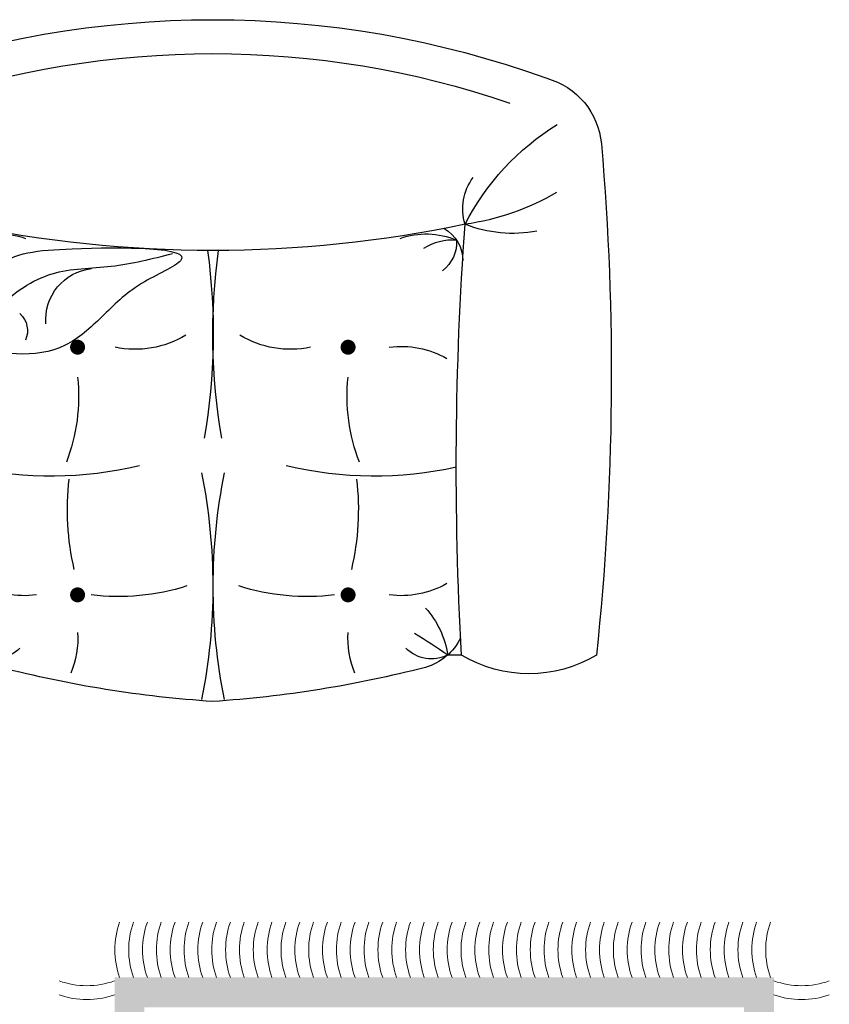
# Model space of a CAD drawing. Units: inches. Extents: x 844 to 2234, y 346 to 1084.
# Tile 63 of 93: x 1860.31 to 1877.53, y 712.91 to 733.85. Entities that reach past the tile are written whole.
import ezdxf

# ---------------------------------------------------------------- set-up
doc = ezdxf.new("R2010")
doc.units = ezdxf.units.IN
doc.header["$MEASUREMENT"] = 0
doc.layers.add('furniture', color=8, linetype='Continuous', lineweight=18)
doc.layers.add('RA-AP-01$0$INT', color=35, linetype='Continuous', lineweight=5)
doc.layers.add('RA-AP-01$0$FURN', color=3, linetype='Continuous')
doc.layers.add('RA-AP-01$0$WOOD', color=64, linetype='Continuous')

# ---------------------------------------------------------------- blocks, each defined once
blk = doc.blocks.new('A$C18D01794')
at = {"layer": 'RA-AP-01$0$INT'}
h = blk.add_hatch(color=256, dxfattribs=at)
h.paths.add_polyline_path([(4.355206456958071, -6.156712009588037), (4.355206456958071, -8.056712009588038), (5.455206456958072, -8.056712009588038), (5.455206456958072, -6.156712009588037)])
h.paths.add_polyline_path([(4.405206456958072, -8.006712009588039), (4.405206456958072, -6.206712009588038), (5.405206456958072, -6.206712009588038), (5.405206456958072, -8.006712009588039)], flags=16)
for centre, start, end in [((4.309006456945037, -8.156264458284674), 70.20384312815696, 109.7961568705686), ((5.501406456971106, -8.156264458284674), 70.20384312943132, 109.796156871843), ((4.309006456945037, -8.179364458283423), 70.20384312815696, 109.7961568705686), ((5.501406456971106, -8.179364458283423), 70.20384312943132, 109.796156871843), ((4.492158905671144, -8.102912009578965), 160.2038431286875, 199.7961568711004), ((4.515258905666937, -8.102912009582035), 160.2038431286875, 199.7961568711004), ((4.53835890566273, -8.102912009585104), 160.2038431286875, 199.7961568711004), ((4.561458905665799, -8.102912009585218), 160.2038431286875, 199.7961568711004), ((4.584558905661592, -8.102912009588287), 160.2038431286875, 199.7961568711004), ((4.607658905664661, -8.102912009588401), 160.2038431286875, 199.7961568711004), ((4.630758905664774, -8.102912009585673), 160.2038431286875, 199.7961568711004), ((4.653858905660567, -8.102912009588742), 160.2038431286875, 199.7961568711004), ((4.676958905663636, -8.102912009588856), 160.2038431286875, 199.7961568711004), ((4.700058905663976, -8.102912009589083), 160.2038431286875, 199.7961568711004), ((4.723158905662498, -8.102912009586241), 160.2038431286875, 199.7961568711004), ((4.746258905662839, -8.102912009586355), 160.2038431286875, 199.7961568711004), ((4.769358905662952, -8.102912009589536), 160.2038431286875, 199.7961568711004), ((4.792458905660109, -8.102912009586696), 160.2038431286875, 199.7961568711004), ((4.815558905661814, -8.10291200958681), 160.2038431286875, 199.7961568711004), ((4.838658905662154, -8.102912009587037), 160.2038431286875, 199.7961568711004), ((4.861758905665223, -8.102912009590106), 160.2038431286875, 199.7961568711004), ((4.884858905661016, -8.102912009587264), 160.2038431286875, 199.7961568711004), ((4.907958905662721, -8.102912009587492), 160.2038431286875, 199.7961568711004), ((4.931058905658514, -8.102912009590447), 160.2038431286875, 199.7961568711004), ((4.954158905661583, -8.102912009587717), 160.2038431286875, 199.7961568711004), ((4.977258905663288, -8.102912009587946), 160.2038431286875, 199.7961568711004), ((5.000358905663628, -8.102912009587946), 160.2038431286875, 199.7961568711004), ((5.023458905665333, -8.10291200959113), 160.2038431286875, 199.7961568711004), ((5.046558905660899, -8.102912009588287), 160.2038431286875, 199.7961568711004), ((5.069658905661239, -8.102912009588401), 160.2038431286875, 199.7961568711004), ((5.092758905664308, -8.102912009588628), 160.2038431286875, 199.7961568711004), ((5.115858905663057, -8.102912009585786), 160.2038431286875, 199.7961568711004), ((5.13895890566317, -8.102912009588856), 160.2038431286875, 199.7961568711004), ((5.162058905663511, -8.102912009589083), 160.2038431286875, 199.7961568711004), ((5.185158905659076, -8.102912009589197), 160.2038431286875, 199.7961568711004), ((5.208258905660781, -8.102912009586355), 160.2038431286875, 199.7961568711004), ((5.231358905662486, -8.102912009589536), 160.2038431286875, 199.7961568711004), ((5.254458905661235, -8.102912009589652), 160.2038431286875, 199.7961568711004), ((5.277558905661575, -8.102912009589765), 160.2038431286875, 199.7961568711004), ((5.300658905661689, -8.102912009587037), 160.2038431286875, 199.7961568711004), ((5.323758905658846, -8.10291200958715), 160.2038431286875, 199.7961568711004), ((5.346858905659186, -8.10291200959022), 160.2038431286875, 199.7961568711004), ((5.369958905662255, -8.102912009587492), 160.2038431286875, 199.7961568711004), ((5.39305890566396, -8.102912009587492), 160.2038431286875, 199.7961568711004), ((5.416158905664301, -8.102912009587717), 160.2038431286875, 199.7961568711004), ((5.439258905666005, -8.102912009590902), 160.2038431286875, 199.7961568711004), ((5.462358905661571, -8.102912009587946), 160.2038431286875, 199.7961568711004), ((5.485458905657364, -8.10291200958499), 160.2038431286875, 199.7961568711004), ((5.508558905660433, -8.102912009588287), 160.2038431286875, 199.7961568711004), ((5.531658905655999, -8.102912009585332), 160.2038431286875, 199.7961568711004), ((5.554758905651792, -8.102912009582376), 160.2038431286875, 199.7961568711004), ((5.577858905654861, -8.102912009585673), 160.2038431286875, 199.7961568711004)]:
    blk.add_arc(centre, 0.136414042854523, start, end, dxfattribs=at)
blk = doc.blocks.new('A$C7F4351E2')
at = {"layer": 'RA-AP-01$0$FURN'}
for p, q in [((8.352559572600457, -8.263941955512525), (8.35255957259913, -8.282283310927069)), ((8.352559572600457, -8.927748273106442), (8.35255957259913, -8.909406917691898))]:
    blk.add_line(p, q, dxfattribs=at)
at = {"layer": 'RA-AP-01$0$FURN', "const_width": 0.01}
for points in [[(8.437812509519787, -8.415359762755768, 1), (8.427812509519786, -8.415359762755742, 1)], [(8.758197489244363, -8.415359762756214, -1), (8.768197489244365, -8.415359762756214, -1)], [(8.437812509519787, -8.776330465863198, -1), (8.427812509519786, -8.776330465863225, -1)], [(8.758197489244363, -8.776330465862753, 1), (8.768197489244365, -8.776330465862753, 1)]]:
    blk.add_lwpolyline(points, format="xyb", close=True, dxfattribs=at)
at = {"layer": 'RA-AP-01$0$FURN'}
for centre, radius, start, end in [((8.727559572604601, -11.61690445537682), 3.552808610866049, 85.0473312316413, 96.05887237565803), ((9.025650106946005, -8.176987401637472), 0.1, 15.499494600857, 85.04733123164159), ((8.50205957259015, -8.17394195551301), 0.1744999999876311, 148.9517780040467, 211.048221995953), ((8.77247054904813, -7.958543863781743), 0.3382138395168437, 297.2303327094027, 328.2563708342649), ((9.2484631175852, -8.302692737637487), 0.3241573581843151, 149.2985674842688, 172.3026350986055), ((7.88981694267423, -8.595845114309485), 1.310286319972027, 340.1192502251003, 19.8807497748998), ((9.084915705374858, -8.196040134964925), 0.1698955038956699, 168.877843135945, 201.8512383801196), ((7.929864357850293, -8.595845114309483), 1.224941341589781, 341.1257460634955, 18.87425393650447), ((8.947672844970796, -8.191835192646359), 0.0704710051510922, 253.1338634205325, 306.4126496157095), ((8.603635103111959, -3.79706073025477), 4.473931917517753, 266.7828902523826, 274.1477233631118), ((10.52713941284929, -8.595845114309466), 1.634931324962266, 168.1200364254424, 191.8799635745573), ((8.408522229993444, -8.33300072568355), 0.0753785023123622, 115.8745619060558, 163.9833547230034), ((9.101231010340802, -8.38034106221356), 0.5100538472773755, 167.6182489359307, 193.3122231353938), ((8.903279781571525, -8.31837865610295), 0.0478550828899777, 86.575295631534, 142.6833829238214), ((8.878389979098333, -8.312202545234353), 0.05, 30.14777190425723, 89.99999999905349), ((8.838100984994732, -8.276822957859652), 0.0683206773889159, 326.6729861493449, 5.218395042636973), ((8.810121490949696, -8.31110757721543), 0.1042084262671507, 340.4828318717155, 22.86929393278168), ((8.395364730619693, -8.304213854581548), 0.0479292786975047, 152.8070868543555, 225.4025460716553), ((8.333592787569726, -8.402663469525104), 0.1218651776285568, 48.0375529564433, 81.04623209541253), ((7.439612310514541, -8.913795367824825), 1.11020813118073, 31.93286085977143, 34.66647731879807), ((8.553131949433, -8.344109762755968), 0.1214118203512435, 150.1419074485596, 187.691663289156), ((8.642878049331348, -8.344109762756093), 0.1214118203512435, 352.3083367106845, 29.85809255128089), ((9.82633505008426, -8.696671375220811), 1.539060359583382, 165.5338783218257, 176.2437734318419), ((8.374918524725835, -8.294321202996931), 0.1212957045587361, 247.3375839744822, 273.7314750942433), ((8.546954810732721, -8.753394424755975), 0.3517162425384579, 83.41248966761125, 103.1674570565571), ((8.697701155637269, -8.172468128267624), 0.2442261434243043, 248.9017070735605, 275.9923925191661), ((8.73287643248165, -8.469775898206471), 0.3023568492824586, 173.0944825511667, 197.588060785551), ((8.889871101981017, -8.492307869305423), 0.1295083186917369, 167.9901339202812, 211.3796151021958), ((8.444145567704187, -7.829943385268752), 0.765467899454341, 258.6273206109321, 281.4174148186357), ((8.781211457338294, -7.772561243483908), 0.8232838708255751, 260.2449188973366, 277.7495311655964), ((9.82633505008426, -8.495018853398156), 1.539060359583382, 183.7562265681581, 194.4661216781742), ((8.444145567704187, -9.361312955433425), 0.765467899454341, 78.58258518136427, 101.3726793890678), ((8.781211457338294, -9.418695097218269), 0.8232838708255751, 82.25060502413102, 99.75508110266344), ((8.73287643248165, -8.721914330412496), 0.3023568492824586, 162.411939214449, 186.9055174488332), ((8.889871101981017, -8.699382359313544), 0.1295083186917369, 148.6203848978042, 192.0098660797188), ((9.101231010340802, -8.811349166405407), 0.5100538472773755, 166.6877768646062, 192.3817510640693), ((8.799643412436344, -8.749969313933361), 0.0689028341546707, 265.5384273543114, 353.5804828909086), ((8.374918524725835, -8.897369025622035), 0.1212957045587361, 86.26852490575668, 112.6624160255178), ((8.546954810732721, -8.438295803862992), 0.3517162425384579, 256.8325429434429, 276.5875103323888), ((8.697701155637269, -9.019222100351342), 0.2442261434243043, 84.00760748083387, 111.0982929264395), ((8.553131949433, -8.847580465862999), 0.1214118203512435, 172.308336710844, 209.8580925514404), ((8.785133372574222, -8.874256642962408), 0.0310151388417235, 42.62105484496073, 114.2239681486109), ((8.810121490949696, -8.880582651403534), 0.1042084262671507, 337.1307060672183, 19.51716812828453), ((8.395364730619693, -8.88747637403742), 0.0479292786975047, 134.5974539283447, 207.1929131456445), ((7.439612310514541, -8.277894860794142), 1.11020813118073, 325.333522681202, 328.0671391402286), ((8.838100984994732, -8.914867270759315), 0.0683206773889159, 354.781604957363, 33.32701385065517), ((8.408522229993444, -8.858689502935416), 0.0753785023123622, 196.0166452769965, 244.1254380939442), ((8.333592787569726, -8.789026759093863), 0.1218651776285568, 278.9537679045875, 311.9624470435567), ((8.642878049331348, -8.847580465862874), 0.1214118203512435, 330.1419074487191, 340.3913536181062), ((8.903279781571525, -8.873311572516016), 0.0478550828899777, 217.3166170761785, 273.424704368466), ((8.878389979098333, -8.879487683384612), 0.05, 270.0000000009465, 337.4173275753961), ((8.50205957259015, -9.017748273105955), 0.1744999999876311, 148.9517780040469, 211.0482219959533), ((8.603635103111959, -13.39462949836419), 4.473931917517753, 85.85227663688822, 93.21710974761734), ((8.947672844970796, -8.999855035972608), 0.0704710051510922, 53.58735038429053, 106.8661365794674), ((9.084915705374858, -8.995650093654042), 0.1698955038956699, 158.1487616198804, 191.122156864055), ((8.77247054904813, -9.233146364837223), 0.3382138395168437, 31.74362916573515, 62.76966729059727), ((9.2484631175852, -8.88899749098148), 0.3241573581843151, 187.6973649013944, 210.7014325157311), ((9.025650106946005, -9.014702826981493), 0.1, 274.9526687683584, 344.500505399143), ((8.727559572604601, -5.574785773242145), 3.552808610866049, 263.941127624342, 274.9526687683587)]:
    blk.add_arc(centre, radius, start, end, dxfattribs=at)
for points, knots in [([(8.764421239581775, -8.929562504990262), (8.755250524728652, -8.881106864374377), (8.74196437992213, -8.810906376383404), (8.80604948961138, -8.740469753734786), (8.847474678848357, -8.701097198289744), (8.897142214037096, -8.58322730303861), (8.897091569728207, -8.784804210134517), (8.88612504526093, -8.897825917224484), (8.806539053396843, -8.9185794820093), (8.764421239581775, -8.92956250499026)], [0, 0, 0, 0, 0.1367586589314792, 0.1981301758052368, 0.2677729570689282, 0.3281194902553322, 0.4737578340741565, 0.5765194025309516, 0.6920332287422236, 0.6920332287422236, 0.6920332287422236, 0.6920332287422236]), ([(8.764421239581775, -8.92956250499026), (8.782204778269502, -8.914603263160053), (8.821592007255505, -8.881471326160916), (8.86917941606436, -8.814322636989944), (8.867818990542759, -8.729338202119969), (8.881231406199264, -8.676770566934765), (8.888101821971249, -8.649843164808122)], [0, 0, 0, 0, 0.070018540671015, 0.1550780383534498, 0.2344491945777043, 0.3178048737568289, 0.3178048737568289, 0.3178048737568289, 0.3178048737568289])]:
    blk.add_open_spline(points, degree=3, knots=knots, dxfattribs=at)
blk = doc.blocks.new('A$C5D2F253E')
at = {"layer": 'RA-AP-01$0$FURN', "xscale": -0.7999999999883585, "yscale": 0.7999999999883585, "zscale": 0.8, "rotation": 90}
blk.add_blockref('A$C18D01794', (-5.687757199772477, 4.75791982714071), dxfattribs=at)
at = {"layer": 'RA-AP-01$0$WOOD', "xscale": -1, "rotation": 180}
blk.add_blockref('A$C7F4351E2', (-7.164808785335935, -7.45332973198748), dxfattribs=at)

msp = doc.modelspace()

# ---------------------------------------------------------------- block references
at = {"layer": 'furniture', "xscale": 15.94108302203742, "yscale": 15.94108302203742, "zscale": 15.94108302203742, "rotation": 90}
msp.add_blockref('A$C5D2F253E', (1882.631064852549, 701.4028671565849), dxfattribs=at)

doc.saveas('drawing.dxf')
